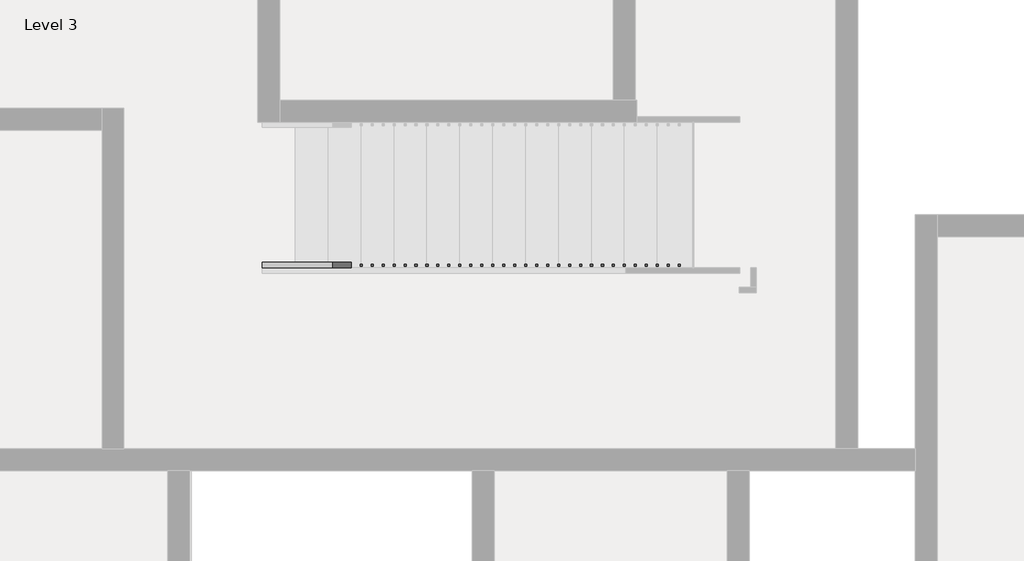
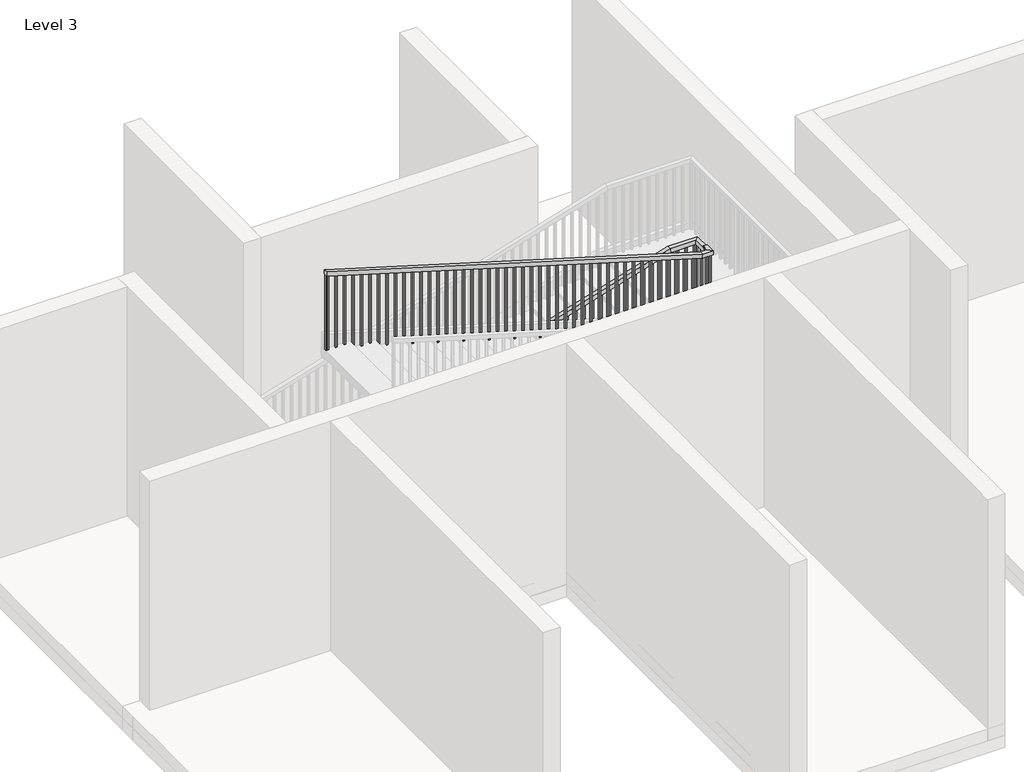
# One storey, part 11 of 14: 1 railing.
"""IFC4 building model written with IfcOpenShell, lengths in millimetres."""

from ifc_helpers import new_model, si_unit, frame, origin, place, context, project, spatial, polyline, outline, extrude, faceted_brep, element, save

model = new_model("IFC4")

# Units and contexts
model_context = context("Model", 3, world=origin())
ifc_project = project(units=[si_unit("LENGTHUNIT", "METRE", prefix="MILLI")], contexts=[model_context])

# Site, building, storey
site = spatial("IfcSite", under=ifc_project)
building = spatial("IfcBuilding", under=site)
storey = spatial("IfcBuildingStorey", under=building, Name="Level 3", Elevation=6096.0)

# Railing
placement = place(None, origin())
element("IfcRailing", 1, ObjectType="Handrail - Rectangular", at=placement, inside=storey, context=model_context, shape_type="SolidModel", body=[
    faceted_brep([(-5254.0891351, 11205.0082924, 7101.84), (-5254.0891351, 11205.0082924, 7048.8032429), (-5254.0891351, 11154.2082924, 7048.8032429), (-5254.0891351, 11154.2082924, 7101.84), (-986.8891351, 11205.0082924, 8382.0), (-979.4332782, 11205.0082924, 8331.2), (-979.4332782, 11154.2082924, 8331.2), (-986.8891351, 11154.2082924, 8382.0), (-631.2891351, 11205.0082924, 8382.0), (-631.2891351, 11205.0082924, 8331.2), (-682.0891351, 11154.2082924, 8331.2), (-682.0891351, 11154.2082924, 8382.0), (-631.2891351, 11001.8082924, 8382.0), (-631.2891351, 10951.0082924, 8331.2), (-682.0891351, 10951.0082924, 8331.2), (-682.0891351, 11001.8082924, 8382.0), (-631.2891351, 11001.8082924, 8404.86), (-631.2891351, 10951.0082924, 8354.06), (-682.0891351, 10951.0082924, 8354.06), (-682.0891351, 11001.8082924, 8404.86), (-631.2891351, 10874.8082924, 8404.86), (-631.2891351, 10874.8082924, 8354.06), (-682.0891351, 10925.6082924, 8354.06), (-682.0891351, 10925.6082924, 8404.86), (-758.2891351, 10874.8082924, 8404.86), (-765.744992, 10874.8082924, 8354.06), (-765.744992, 10925.6082924, 8354.06), (-758.2891351, 10925.6082924, 8404.86), (-5254.0891351, 10874.8082924, 9753.6), (-5254.0891351, 10925.6082924, 9753.6), (-5254.0891351, 10925.6082924, 9700.5632429), (-5254.0891351, 10874.8082924, 9700.5632429)], [[[0, 1, 2, 3]], [[1, 0, 4, 5]], [[2, 1, 5, 6]], [[3, 2, 6, 7]], [[0, 3, 7, 4]], [[5, 4, 8, 9]], [[6, 5, 9, 10]], [[7, 6, 10, 11]], [[4, 7, 11, 8]], [[9, 8, 12, 13]], [[10, 9, 13, 14]], [[11, 10, 14, 15]], [[8, 11, 15, 12]], [[13, 12, 16, 17]], [[14, 13, 17, 18]], [[15, 14, 18, 19]], [[12, 15, 19, 16]], [[17, 16, 20, 21]], [[18, 17, 21, 22]], [[19, 18, 22, 23]], [[16, 19, 23, 20]], [[21, 20, 24, 25]], [[22, 21, 25, 26]], [[23, 22, 26, 27]], [[20, 23, 27, 24]], [[28, 29, 30, 31]], [[25, 24, 28, 31]], [[26, 25, 31, 30]], [[27, 26, 30, 29]], [[24, 27, 29, 28]]]),
    extrude(outline(polyline([(9690.0857429, -5219.1641351), (9695.8007429, -5238.2141351), (8747.76, -5238.2141351), (8747.76, -5219.1641351), (9690.0857429, -5219.1641351)])), frame((0.0, 10890.6832924, 0.0), z_axis=(0.0, 1.0, 0.0), x_axis=(0.0, 0.0, 1.0)), (0.0, 0.0, 1.0), 19.05),
    extrude(outline(polyline([(9659.6057429, -5117.5641351), (9665.3207429, -5136.6141351), (8747.76, -5136.6141351), (8747.76, -5117.5641351), (9659.6057429, -5117.5641351)])), frame((0.0, 10890.6832924, 0.0), z_axis=(0.0, 1.0, 0.0), x_axis=(0.0, 0.0, 1.0)), (0.0, 0.0, 1.0), 19.05),
    extrude(outline(polyline([(9629.1257429, -5015.9641351), (9634.8407429, -5035.0141351), (8747.76, -5035.0141351), (8747.76, -5015.9641351), (9629.1257429, -5015.9641351)])), frame((0.0, 10890.6832924, 0.0), z_axis=(0.0, 1.0, 0.0), x_axis=(0.0, 0.0, 1.0)), (0.0, 0.0, 1.0), 19.05),
    extrude(outline(polyline([(9598.6457429, -4914.3641351), (9604.3607429, -4933.4141351), (8656.32, -4933.4141351), (8656.32, -4914.3641351), (9598.6457429, -4914.3641351)])), frame((0.0, 10890.6832924, 0.0), z_axis=(0.0, 1.0, 0.0), x_axis=(0.0, 0.0, 1.0)), (0.0, 0.0, 1.0), 19.05),
    extrude(outline(polyline([(9568.1657429, -4812.7641351), (9573.8807429, -4831.8141351), (8656.32, -4831.8141351), (8656.32, -4812.7641351), (9568.1657429, -4812.7641351)])), frame((0.0, 10890.6832924, 0.0), z_axis=(0.0, 1.0, 0.0), x_axis=(0.0, 0.0, 1.0)), (0.0, 0.0, 1.0), 19.05),
    extrude(outline(polyline([(9537.6857429, -4711.1641351), (9543.4007429, -4730.2141351), (8656.32, -4730.2141351), (8656.32, -4711.1641351), (9537.6857429, -4711.1641351)])), frame((0.0, 10890.6832924, 0.0), z_axis=(0.0, 1.0, 0.0), x_axis=(0.0, 0.0, 1.0)), (0.0, 0.0, 1.0), 19.05),
    extrude(outline(polyline([(9507.2057429, -4609.5641351), (9512.9207429, -4628.6141351), (8564.88, -4628.6141351), (8564.88, -4609.5641351), (9507.2057429, -4609.5641351)])), frame((0.0, 10890.6832924, 0.0), z_axis=(0.0, 1.0, 0.0), x_axis=(0.0, 0.0, 1.0)), (0.0, 0.0, 1.0), 19.05),
    extrude(outline(polyline([(9476.7257429, -4507.9641351), (9482.4407429, -4527.0141351), (8564.88, -4527.0141351), (8564.88, -4507.9641351), (9476.7257429, -4507.9641351)])), frame((0.0, 10890.6832924, 0.0), z_axis=(0.0, 1.0, 0.0), x_axis=(0.0, 0.0, 1.0)), (0.0, 0.0, 1.0), 19.05),
    extrude(outline(polyline([(9446.2457429, -4406.3641351), (9451.9607429, -4425.4141351), (8564.88, -4425.4141351), (8564.88, -4406.3641351), (9446.2457429, -4406.3641351)])), frame((0.0, 10890.6832924, 0.0), z_axis=(0.0, 1.0, 0.0), x_axis=(0.0, 0.0, 1.0)), (0.0, 0.0, 1.0), 19.05),
    extrude(outline(polyline([(9415.7657429, -4304.7641351), (9421.4807429, -4323.8141351), (8473.44, -4323.8141351), (8473.44, -4304.7641351), (9415.7657429, -4304.7641351)])), frame((0.0, 10890.6832924, 0.0), z_axis=(0.0, 1.0, 0.0), x_axis=(0.0, 0.0, 1.0)), (0.0, 0.0, 1.0), 19.05),
    extrude(outline(polyline([(9385.2857429, -4203.1641351), (9391.0007429, -4222.2141351), (8473.44, -4222.2141351), (8473.44, -4203.1641351), (9385.2857429, -4203.1641351)])), frame((0.0, 10890.6832924, 0.0), z_axis=(0.0, 1.0, 0.0), x_axis=(0.0, 0.0, 1.0)), (0.0, 0.0, 1.0), 19.05),
    extrude(outline(polyline([(9354.8057429, -4101.5641351), (9360.5207429, -4120.6141351), (8473.44, -4120.6141351), (8473.44, -4101.5641351), (9354.8057429, -4101.5641351)])), frame((0.0, 10890.6832924, 0.0), z_axis=(0.0, 1.0, 0.0), x_axis=(0.0, 0.0, 1.0)), (0.0, 0.0, 1.0), 19.05),
    extrude(outline(polyline([(9324.3257429, -3999.9641351), (9330.0407429, -4019.0141351), (8382.0, -4019.0141351), (8382.0, -3999.9641351), (9324.3257429, -3999.9641351)])), frame((0.0, 10890.6832924, 0.0), z_axis=(0.0, 1.0, 0.0), x_axis=(0.0, 0.0, 1.0)), (0.0, 0.0, 1.0), 19.05),
    extrude(outline(polyline([(9293.8457429, -3898.3641351), (9299.5607429, -3917.4141351), (8382.0, -3917.4141351), (8382.0, -3898.3641351), (9293.8457429, -3898.3641351)])), frame((0.0, 10890.6832924, 0.0), z_axis=(0.0, 1.0, 0.0), x_axis=(0.0, 0.0, 1.0)), (0.0, 0.0, 1.0), 19.05),
    extrude(outline(polyline([(9263.3657429, -3796.7641351), (9269.0807429, -3815.8141351), (8382.0, -3815.8141351), (8382.0, -3796.7641351), (9263.3657429, -3796.7641351)])), frame((0.0, 10890.6832924, 0.0), z_axis=(0.0, 1.0, 0.0), x_axis=(0.0, 0.0, 1.0)), (0.0, 0.0, 1.0), 19.05),
    extrude(outline(polyline([(9232.8857429, -3695.1641351), (9238.6007429, -3714.2141351), (8290.56, -3714.2141351), (8290.56, -3695.1641351), (9232.8857429, -3695.1641351)])), frame((0.0, 10890.6832924, 0.0), z_axis=(0.0, 1.0, 0.0), x_axis=(0.0, 0.0, 1.0)), (0.0, 0.0, 1.0), 19.05),
    extrude(outline(polyline([(9202.4057429, -3593.5641351), (9208.1207429, -3612.6141351), (8290.56, -3612.6141351), (8290.56, -3593.5641351), (9202.4057429, -3593.5641351)])), frame((0.0, 10890.6832924, 0.0), z_axis=(0.0, 1.0, 0.0), x_axis=(0.0, 0.0, 1.0)), (0.0, 0.0, 1.0), 19.05),
    extrude(outline(polyline([(9171.9257429, -3491.9641351), (9177.6407429, -3511.0141351), (8290.56, -3511.0141351), (8290.56, -3491.9641351), (9171.9257429, -3491.9641351)])), frame((0.0, 10890.6832924, 0.0), z_axis=(0.0, 1.0, 0.0), x_axis=(0.0, 0.0, 1.0)), (0.0, 0.0, 1.0), 19.05),
    extrude(outline(polyline([(9141.4457429, -3390.3641351), (9147.1607429, -3409.4141351), (8199.12, -3409.4141351), (8199.12, -3390.3641351), (9141.4457429, -3390.3641351)])), frame((0.0, 10890.6832924, 0.0), z_axis=(0.0, 1.0, 0.0), x_axis=(0.0, 0.0, 1.0)), (0.0, 0.0, 1.0), 19.05),
    extrude(outline(polyline([(9110.9657429, -3288.7641351), (9116.6807429, -3307.8141351), (8199.12, -3307.8141351), (8199.12, -3288.7641351), (9110.9657429, -3288.7641351)])), frame((0.0, 10890.6832924, 0.0), z_axis=(0.0, 1.0, 0.0), x_axis=(0.0, 0.0, 1.0)), (0.0, 0.0, 1.0), 19.05),
    extrude(outline(polyline([(9080.4857429, -3187.1641351), (9086.2007429, -3206.2141351), (8199.12, -3206.2141351), (8199.12, -3187.1641351), (9080.4857429, -3187.1641351)])), frame((0.0, 10890.6832924, 0.0), z_axis=(0.0, 1.0, 0.0), x_axis=(0.0, 0.0, 1.0)), (0.0, 0.0, 1.0), 19.05),
    extrude(outline(polyline([(9050.0057429, -3085.5641351), (9055.7207429, -3104.6141351), (8107.68, -3104.6141351), (8107.68, -3085.5641351), (9050.0057429, -3085.5641351)])), frame((0.0, 10890.6832924, 0.0), z_axis=(0.0, 1.0, 0.0), x_axis=(0.0, 0.0, 1.0)), (0.0, 0.0, 1.0), 19.05),
    extrude(outline(polyline([(9019.5257429, -2983.9641351), (9025.2407429, -3003.0141351), (8107.68, -3003.0141351), (8107.68, -2983.9641351), (9019.5257429, -2983.9641351)])), frame((0.0, 10890.6832924, 0.0), z_axis=(0.0, 1.0, 0.0), x_axis=(0.0, 0.0, 1.0)), (0.0, 0.0, 1.0), 19.05),
    extrude(outline(polyline([(8989.0457429, -2882.3641351), (8994.7607429, -2901.4141351), (8107.68, -2901.4141351), (8107.68, -2882.3641351), (8989.0457429, -2882.3641351)])), frame((0.0, 10890.6832924, 0.0), z_axis=(0.0, 1.0, 0.0), x_axis=(0.0, 0.0, 1.0)), (0.0, 0.0, 1.0), 19.05),
    extrude(outline(polyline([(8958.5657429, -2780.7641351), (8964.2807429, -2799.8141351), (8016.24, -2799.8141351), (8016.24, -2780.7641351), (8958.5657429, -2780.7641351)])), frame((0.0, 10890.6832924, 0.0), z_axis=(0.0, 1.0, 0.0), x_axis=(0.0, 0.0, 1.0)), (0.0, 0.0, 1.0), 19.05),
    extrude(outline(polyline([(8928.0857429, -2679.1641351), (8933.8007429, -2698.2141351), (8016.24, -2698.2141351), (8016.24, -2679.1641351), (8928.0857429, -2679.1641351)])), frame((0.0, 10890.6832924, 0.0), z_axis=(0.0, 1.0, 0.0), x_axis=(0.0, 0.0, 1.0)), (0.0, 0.0, 1.0), 19.05),
    extrude(outline(polyline([(8897.6057429, -2577.5641351), (8903.3207429, -2596.6141351), (8016.24, -2596.6141351), (8016.24, -2577.5641351), (8897.6057429, -2577.5641351)])), frame((0.0, 10890.6832924, 0.0), z_axis=(0.0, 1.0, 0.0), x_axis=(0.0, 0.0, 1.0)), (0.0, 0.0, 1.0), 19.05),
    extrude(outline(polyline([(8867.1257429, -2475.9641351), (8872.8407429, -2495.0141351), (7924.8, -2495.0141351), (7924.8, -2475.9641351), (8867.1257429, -2475.9641351)])), frame((0.0, 10890.6832924, 0.0), z_axis=(0.0, 1.0, 0.0), x_axis=(0.0, 0.0, 1.0)), (0.0, 0.0, 1.0), 19.05),
    extrude(outline(polyline([(8836.6457429, -2374.3641351), (8842.3607429, -2393.4141351), (7924.8, -2393.4141351), (7924.8, -2374.3641351), (8836.6457429, -2374.3641351)])), frame((0.0, 10890.6832924, 0.0), z_axis=(0.0, 1.0, 0.0), x_axis=(0.0, 0.0, 1.0)), (0.0, 0.0, 1.0), 19.05),
    extrude(outline(polyline([(8806.1657429, -2272.7641351), (8811.8807429, -2291.8141351), (7924.8, -2291.8141351), (7924.8, -2272.7641351), (8806.1657429, -2272.7641351)])), frame((0.0, 10890.6832924, 0.0), z_axis=(0.0, 1.0, 0.0), x_axis=(0.0, 0.0, 1.0)), (0.0, 0.0, 1.0), 19.05),
    extrude(outline(polyline([(8775.6857429, -2171.1641351), (8781.4007429, -2190.2141351), (7833.36, -2190.2141351), (7833.36, -2171.1641351), (8775.6857429, -2171.1641351)])), frame((0.0, 10890.6832924, 0.0), z_axis=(0.0, 1.0, 0.0), x_axis=(0.0, 0.0, 1.0)), (0.0, 0.0, 1.0), 19.05),
    extrude(outline(polyline([(8745.2057429, -2069.5641351), (8750.9207429, -2088.6141351), (7833.36, -2088.6141351), (7833.36, -2069.5641351), (8745.2057429, -2069.5641351)])), frame((0.0, 10890.6832924, 0.0), z_axis=(0.0, 1.0, 0.0), x_axis=(0.0, 0.0, 1.0)), (0.0, 0.0, 1.0), 19.05),
    extrude(outline(polyline([(8714.7257429, -1967.9641351), (8720.4407429, -1987.0141351), (7833.36, -1987.0141351), (7833.36, -1967.9641351), (8714.7257429, -1967.9641351)])), frame((0.0, 10890.6832924, 0.0), z_axis=(0.0, 1.0, 0.0), x_axis=(0.0, 0.0, 1.0)), (0.0, 0.0, 1.0), 19.05),
    extrude(outline(polyline([(8684.2457429, -1866.3641351), (8689.9607429, -1885.4141351), (7741.92, -1885.4141351), (7741.92, -1866.3641351), (8684.2457429, -1866.3641351)])), frame((0.0, 10890.6832924, 0.0), z_axis=(0.0, 1.0, 0.0), x_axis=(0.0, 0.0, 1.0)), (0.0, 0.0, 1.0), 19.05),
    extrude(outline(polyline([(8653.7657429, -1764.7641351), (8659.4807429, -1783.8141351), (7741.92, -1783.8141351), (7741.92, -1764.7641351), (8653.7657429, -1764.7641351)])), frame((0.0, 10890.6832924, 0.0), z_axis=(0.0, 1.0, 0.0), x_axis=(0.0, 0.0, 1.0)), (0.0, 0.0, 1.0), 19.05),
    extrude(outline(polyline([(8623.2857429, -1663.1641351), (8629.0007429, -1682.2141351), (7741.92, -1682.2141351), (7741.92, -1663.1641351), (8623.2857429, -1663.1641351)])), frame((0.0, 10890.6832924, 0.0), z_axis=(0.0, 1.0, 0.0), x_axis=(0.0, 0.0, 1.0)), (0.0, 0.0, 1.0), 19.05),
    extrude(outline(polyline([(8592.8057429, -1561.5641351), (8598.5207429, -1580.6141351), (7650.48, -1580.6141351), (7650.48, -1561.5641351), (8592.8057429, -1561.5641351)])), frame((0.0, 10890.6832924, 0.0), z_axis=(0.0, 1.0, 0.0), x_axis=(0.0, 0.0, 1.0)), (0.0, 0.0, 1.0), 19.05),
    extrude(outline(polyline([(8562.3257429, -1459.9641351), (8568.0407429, -1479.0141351), (7650.48, -1479.0141351), (7650.48, -1459.9641351), (8562.3257429, -1459.9641351)])), frame((0.0, 10890.6832924, 0.0), z_axis=(0.0, 1.0, 0.0), x_axis=(0.0, 0.0, 1.0)), (0.0, 0.0, 1.0), 19.05),
    extrude(outline(polyline([(8531.8457429, -1358.3641351), (8537.5607429, -1377.4141351), (7650.48, -1377.4141351), (7650.48, -1358.3641351), (8531.8457429, -1358.3641351)])), frame((0.0, 10890.6832924, 0.0), z_axis=(0.0, 1.0, 0.0), x_axis=(0.0, 0.0, 1.0)), (0.0, 0.0, 1.0), 19.05),
    extrude(outline(polyline([(8501.3657429, -1256.7641351), (8507.0807429, -1275.8141351), (7559.04, -1275.8141351), (7559.04, -1256.7641351), (8501.3657429, -1256.7641351)])), frame((0.0, 10890.6832924, 0.0), z_axis=(0.0, 1.0, 0.0), x_axis=(0.0, 0.0, 1.0)), (0.0, 0.0, 1.0), 19.05),
    extrude(outline(polyline([(8470.8857429, -1155.1641351), (8476.6007429, -1174.2141351), (7559.04, -1174.2141351), (7559.04, -1155.1641351), (8470.8857429, -1155.1641351)])), frame((0.0, 10890.6832924, 0.0), z_axis=(0.0, 1.0, 0.0), x_axis=(0.0, 0.0, 1.0)), (0.0, 0.0, 1.0), 19.05),
    extrude(outline(polyline([(8440.4057429, -1053.5641351), (8446.1207429, -1072.6141351), (7559.04, -1072.6141351), (7559.04, -1053.5641351), (8440.4057429, -1053.5641351)])), frame((0.0, 10890.6832924, 0.0), z_axis=(0.0, 1.0, 0.0), x_axis=(0.0, 0.0, 1.0)), (0.0, 0.0, 1.0), 19.05),
    extrude(outline(polyline([(8409.9257429, -951.9641351), (8415.6407429, -971.0141351), (7467.6, -971.0141351), (7467.6, -951.9641351), (8409.9257429, -951.9641351)])), frame((0.0, 10890.6832924, 0.0), z_axis=(0.0, 1.0, 0.0), x_axis=(0.0, 0.0, 1.0)), (0.0, 0.0, 1.0), 19.05),
    extrude(outline(polyline([(8379.4457429, -850.3641351), (8385.1607429, -869.4141351), (7467.6, -869.4141351), (7467.6, -850.3641351), (8379.4457429, -850.3641351)])), frame((0.0, 10890.6832924, 0.0), z_axis=(0.0, 1.0, 0.0), x_axis=(0.0, 0.0, 1.0)), (0.0, 0.0, 1.0), 19.05),
    extrude(outline(polyline([(8348.9657429, -748.7641351), (8354.6807429, -767.8141351), (7467.6, -767.8141351), (7467.6, -748.7641351), (8348.9657429, -748.7641351)])), frame((0.0, 10890.6832924, 0.0), z_axis=(0.0, 1.0, 0.0), x_axis=(0.0, 0.0, 1.0)), (0.0, 0.0, 1.0), 19.05),
    extrude(outline(polyline([(-666.2141351, 10985.9332924), (-647.1641351, 10985.9332924), (-647.1641351, 10966.8832924), (-666.2141351, 10966.8832924), (-666.2141351, 10985.9332924)])), frame((0.0, 0.0, 7467.6), z_axis=(0.0, 0.0, 1.0), x_axis=(1.0, 0.0, 0.0)), (0.0, 0.0, 1.0), 886.46),
    extrude(outline(polyline([(-666.2141351, 11087.5332924), (-647.1641351, 11087.5332924), (-647.1641351, 11068.4832924), (-666.2141351, 11068.4832924), (-666.2141351, 11087.5332924)])), frame((0.0, 0.0, 7467.6), z_axis=(0.0, 0.0, 1.0), x_axis=(1.0, 0.0, 0.0)), (0.0, 0.0, 1.0), 863.6),
    extrude(outline(polyline([(-691.6141351, 11170.0832924), (-691.6141351, 11189.1332924), (-672.5641351, 11189.1332924), (-672.5641351, 11170.0832924), (-691.6141351, 11170.0832924)])), frame((0.0, 0.0, 7467.6), z_axis=(0.0, 0.0, 1.0), x_axis=(1.0, 0.0, 0.0)), (0.0, 0.0, 1.0), 863.6),
    extrude(outline(polyline([(-793.2141351, 11170.0832924), (-793.2141351, 11189.1332924), (-774.1641351, 11189.1332924), (-774.1641351, 11170.0832924), (-793.2141351, 11170.0832924)])), frame((0.0, 0.0, 7467.6), z_axis=(0.0, 0.0, 1.0), x_axis=(1.0, 0.0, 0.0)), (0.0, 0.0, 1.0), 863.6),
    extrude(outline(polyline([(-894.8141351, 11170.0832924), (-894.8141351, 11189.1332924), (-875.7641351, 11189.1332924), (-875.7641351, 11170.0832924), (-894.8141351, 11170.0832924)])), frame((0.0, 0.0, 7467.6), z_axis=(0.0, 0.0, 1.0), x_axis=(1.0, 0.0, 0.0)), (0.0, 0.0, 1.0), 863.6),
    extrude(outline(polyline([(8331.8207429, -977.3641351), (8326.1057429, -996.4141351), (7467.6, -996.4141351), (7467.6, -977.3641351), (8331.8207429, -977.3641351)])), frame((0.0, 11170.0832924, 0.0), z_axis=(0.0, 1.0, 0.0), x_axis=(0.0, 0.0, 1.0)), (0.0, 0.0, 1.0), 19.05),
    extrude(outline(polyline([(8301.3407429, -1078.9641351), (8295.6257429, -1098.0141351), (7376.16, -1098.0141351), (7376.16, -1078.9641351), (8301.3407429, -1078.9641351)])), frame((0.0, 11170.0832924, 0.0), z_axis=(0.0, 1.0, 0.0), x_axis=(0.0, 0.0, 1.0)), (0.0, 0.0, 1.0), 19.05),
    extrude(outline(polyline([(8270.8607429, -1180.5641351), (8265.1457429, -1199.6141351), (7376.16, -1199.6141351), (7376.16, -1180.5641351), (8270.8607429, -1180.5641351)])), frame((0.0, 11170.0832924, 0.0), z_axis=(0.0, 1.0, 0.0), x_axis=(0.0, 0.0, 1.0)), (0.0, 0.0, 1.0), 19.05),
    extrude(outline(polyline([(8240.3807429, -1282.1641351), (8234.6657429, -1301.2141351), (7376.16, -1301.2141351), (7376.16, -1282.1641351), (8240.3807429, -1282.1641351)])), frame((0.0, 11170.0832924, 0.0), z_axis=(0.0, 1.0, 0.0), x_axis=(0.0, 0.0, 1.0)), (0.0, 0.0, 1.0), 19.05),
    extrude(outline(polyline([(8209.9007429, -1383.7641351), (8204.1857429, -1402.8141351), (7284.72, -1402.8141351), (7284.72, -1383.7641351), (8209.9007429, -1383.7641351)])), frame((0.0, 11170.0832924, 0.0), z_axis=(0.0, 1.0, 0.0), x_axis=(0.0, 0.0, 1.0)), (0.0, 0.0, 1.0), 19.05),
    extrude(outline(polyline([(8179.4207429, -1485.3641351), (8173.7057429, -1504.4141351), (7284.72, -1504.4141351), (7284.72, -1485.3641351), (8179.4207429, -1485.3641351)])), frame((0.0, 11170.0832924, 0.0), z_axis=(0.0, 1.0, 0.0), x_axis=(0.0, 0.0, 1.0)), (0.0, 0.0, 1.0), 19.05),
    extrude(outline(polyline([(8148.9407429, -1586.9641351), (8143.2257429, -1606.0141351), (7284.72, -1606.0141351), (7284.72, -1586.9641351), (8148.9407429, -1586.9641351)])), frame((0.0, 11170.0832924, 0.0), z_axis=(0.0, 1.0, 0.0), x_axis=(0.0, 0.0, 1.0)), (0.0, 0.0, 1.0), 19.05),
    extrude(outline(polyline([(8118.4607429, -1688.5641351), (8112.7457429, -1707.6141351), (7193.28, -1707.6141351), (7193.28, -1688.5641351), (8118.4607429, -1688.5641351)])), frame((0.0, 11170.0832924, 0.0), z_axis=(0.0, 1.0, 0.0), x_axis=(0.0, 0.0, 1.0)), (0.0, 0.0, 1.0), 19.05),
    extrude(outline(polyline([(8087.9807429, -1790.1641351), (8082.2657429, -1809.2141351), (7193.28, -1809.2141351), (7193.28, -1790.1641351), (8087.9807429, -1790.1641351)])), frame((0.0, 11170.0832924, 0.0), z_axis=(0.0, 1.0, 0.0), x_axis=(0.0, 0.0, 1.0)), (0.0, 0.0, 1.0), 19.05),
    extrude(outline(polyline([(8057.5007429, -1891.7641351), (8051.7857429, -1910.8141351), (7193.28, -1910.8141351), (7193.28, -1891.7641351), (8057.5007429, -1891.7641351)])), frame((0.0, 11170.0832924, 0.0), z_axis=(0.0, 1.0, 0.0), x_axis=(0.0, 0.0, 1.0)), (0.0, 0.0, 1.0), 19.05),
    extrude(outline(polyline([(8027.0207429, -1993.3641351), (8021.3057429, -2012.4141351), (7101.84, -2012.4141351), (7101.84, -1993.3641351), (8027.0207429, -1993.3641351)])), frame((0.0, 11170.0832924, 0.0), z_axis=(0.0, 1.0, 0.0), x_axis=(0.0, 0.0, 1.0)), (0.0, 0.0, 1.0), 19.05),
    extrude(outline(polyline([(7996.5407429, -2094.9641351), (7990.8257429, -2114.0141351), (7101.84, -2114.0141351), (7101.84, -2094.9641351), (7996.5407429, -2094.9641351)])), frame((0.0, 11170.0832924, 0.0), z_axis=(0.0, 1.0, 0.0), x_axis=(0.0, 0.0, 1.0)), (0.0, 0.0, 1.0), 19.05),
    extrude(outline(polyline([(7966.0607429, -2196.5641351), (7960.3457429, -2215.6141351), (7101.84, -2215.6141351), (7101.84, -2196.5641351), (7966.0607429, -2196.5641351)])), frame((0.0, 11170.0832924, 0.0), z_axis=(0.0, 1.0, 0.0), x_axis=(0.0, 0.0, 1.0)), (0.0, 0.0, 1.0), 19.05),
    extrude(outline(polyline([(7935.5807429, -2298.1641351), (7929.8657429, -2317.2141351), (7010.4, -2317.2141351), (7010.4, -2298.1641351), (7935.5807429, -2298.1641351)])), frame((0.0, 11170.0832924, 0.0), z_axis=(0.0, 1.0, 0.0), x_axis=(0.0, 0.0, 1.0)), (0.0, 0.0, 1.0), 19.05),
    extrude(outline(polyline([(7905.1007429, -2399.7641351), (7899.3857429, -2418.8141351), (7010.4, -2418.8141351), (7010.4, -2399.7641351), (7905.1007429, -2399.7641351)])), frame((0.0, 11170.0832924, 0.0), z_axis=(0.0, 1.0, 0.0), x_axis=(0.0, 0.0, 1.0)), (0.0, 0.0, 1.0), 19.05),
    extrude(outline(polyline([(7874.6207429, -2501.3641351), (7868.9057429, -2520.4141351), (7010.4, -2520.4141351), (7010.4, -2501.3641351), (7874.6207429, -2501.3641351)])), frame((0.0, 11170.0832924, 0.0), z_axis=(0.0, 1.0, 0.0), x_axis=(0.0, 0.0, 1.0)), (0.0, 0.0, 1.0), 19.05),
    extrude(outline(polyline([(7844.1407429, -2602.9641351), (7838.4257429, -2622.0141351), (6918.96, -2622.0141351), (6918.96, -2602.9641351), (7844.1407429, -2602.9641351)])), frame((0.0, 11170.0832924, 0.0), z_axis=(0.0, 1.0, 0.0), x_axis=(0.0, 0.0, 1.0)), (0.0, 0.0, 1.0), 19.05),
    extrude(outline(polyline([(7813.6607429, -2704.5641351), (7807.9457429, -2723.6141351), (6918.96, -2723.6141351), (6918.96, -2704.5641351), (7813.6607429, -2704.5641351)])), frame((0.0, 11170.0832924, 0.0), z_axis=(0.0, 1.0, 0.0), x_axis=(0.0, 0.0, 1.0)), (0.0, 0.0, 1.0), 19.05),
    extrude(outline(polyline([(7783.1807429, -2806.1641351), (7777.4657429, -2825.2141351), (6918.96, -2825.2141351), (6918.96, -2806.1641351), (7783.1807429, -2806.1641351)])), frame((0.0, 11170.0832924, 0.0), z_axis=(0.0, 1.0, 0.0), x_axis=(0.0, 0.0, 1.0)), (0.0, 0.0, 1.0), 19.05),
    extrude(outline(polyline([(7752.7007429, -2907.7641351), (7746.9857429, -2926.8141351), (6827.52, -2926.8141351), (6827.52, -2907.7641351), (7752.7007429, -2907.7641351)])), frame((0.0, 11170.0832924, 0.0), z_axis=(0.0, 1.0, 0.0), x_axis=(0.0, 0.0, 1.0)), (0.0, 0.0, 1.0), 19.05),
    extrude(outline(polyline([(7722.2207429, -3009.3641351), (7716.5057429, -3028.4141351), (6827.52, -3028.4141351), (6827.52, -3009.3641351), (7722.2207429, -3009.3641351)])), frame((0.0, 11170.0832924, 0.0), z_axis=(0.0, 1.0, 0.0), x_axis=(0.0, 0.0, 1.0)), (0.0, 0.0, 1.0), 19.05),
    extrude(outline(polyline([(7691.7407429, -3110.9641351), (7686.0257429, -3130.0141351), (6827.52, -3130.0141351), (6827.52, -3110.9641351), (7691.7407429, -3110.9641351)])), frame((0.0, 11170.0832924, 0.0), z_axis=(0.0, 1.0, 0.0), x_axis=(0.0, 0.0, 1.0)), (0.0, 0.0, 1.0), 19.05),
    extrude(outline(polyline([(7661.2607429, -3212.5641351), (7655.5457429, -3231.6141351), (6736.08, -3231.6141351), (6736.08, -3212.5641351), (7661.2607429, -3212.5641351)])), frame((0.0, 11170.0832924, 0.0), z_axis=(0.0, 1.0, 0.0), x_axis=(0.0, 0.0, 1.0)), (0.0, 0.0, 1.0), 19.05),
    extrude(outline(polyline([(7630.7807429, -3314.1641351), (7625.0657429, -3333.2141351), (6736.08, -3333.2141351), (6736.08, -3314.1641351), (7630.7807429, -3314.1641351)])), frame((0.0, 11170.0832924, 0.0), z_axis=(0.0, 1.0, 0.0), x_axis=(0.0, 0.0, 1.0)), (0.0, 0.0, 1.0), 19.05),
    extrude(outline(polyline([(7600.3007429, -3415.7641351), (7594.5857429, -3434.8141351), (6736.08, -3434.8141351), (6736.08, -3415.7641351), (7600.3007429, -3415.7641351)])), frame((0.0, 11170.0832924, 0.0), z_axis=(0.0, 1.0, 0.0), x_axis=(0.0, 0.0, 1.0)), (0.0, 0.0, 1.0), 19.05),
    extrude(outline(polyline([(7569.8207429, -3517.3641351), (7564.1057429, -3536.4141351), (6644.64, -3536.4141351), (6644.64, -3517.3641351), (7569.8207429, -3517.3641351)])), frame((0.0, 11170.0832924, 0.0), z_axis=(0.0, 1.0, 0.0), x_axis=(0.0, 0.0, 1.0)), (0.0, 0.0, 1.0), 19.05),
    extrude(outline(polyline([(7539.3407429, -3618.9641351), (7533.6257429, -3638.0141351), (6644.64, -3638.0141351), (6644.64, -3618.9641351), (7539.3407429, -3618.9641351)])), frame((0.0, 11170.0832924, 0.0), z_axis=(0.0, 1.0, 0.0), x_axis=(0.0, 0.0, 1.0)), (0.0, 0.0, 1.0), 19.05),
    extrude(outline(polyline([(7508.8607429, -3720.5641351), (7503.1457429, -3739.6141351), (6644.64, -3739.6141351), (6644.64, -3720.5641351), (7508.8607429, -3720.5641351)])), frame((0.0, 11170.0832924, 0.0), z_axis=(0.0, 1.0, 0.0), x_axis=(0.0, 0.0, 1.0)), (0.0, 0.0, 1.0), 19.05),
    extrude(outline(polyline([(7478.3807429, -3822.1641351), (7472.6657429, -3841.2141351), (6553.2, -3841.2141351), (6553.2, -3822.1641351), (7478.3807429, -3822.1641351)])), frame((0.0, 11170.0832924, 0.0), z_axis=(0.0, 1.0, 0.0), x_axis=(0.0, 0.0, 1.0)), (0.0, 0.0, 1.0), 19.05),
    extrude(outline(polyline([(7447.9007429, -3923.7641351), (7442.1857429, -3942.8141351), (6553.2, -3942.8141351), (6553.2, -3923.7641351), (7447.9007429, -3923.7641351)])), frame((0.0, 11170.0832924, 0.0), z_axis=(0.0, 1.0, 0.0), x_axis=(0.0, 0.0, 1.0)), (0.0, 0.0, 1.0), 19.05),
    extrude(outline(polyline([(7417.4207429, -4025.3641351), (7411.7057429, -4044.4141351), (6553.2, -4044.4141351), (6553.2, -4025.3641351), (7417.4207429, -4025.3641351)])), frame((0.0, 11170.0832924, 0.0), z_axis=(0.0, 1.0, 0.0), x_axis=(0.0, 0.0, 1.0)), (0.0, 0.0, 1.0), 19.05),
    extrude(outline(polyline([(7386.9407429, -4126.9641351), (7381.2257429, -4146.0141351), (6461.76, -4146.0141351), (6461.76, -4126.9641351), (7386.9407429, -4126.9641351)])), frame((0.0, 11170.0832924, 0.0), z_axis=(0.0, 1.0, 0.0), x_axis=(0.0, 0.0, 1.0)), (0.0, 0.0, 1.0), 19.05),
    extrude(outline(polyline([(7356.4607429, -4228.5641351), (7350.7457429, -4247.6141351), (6461.76, -4247.6141351), (6461.76, -4228.5641351), (7356.4607429, -4228.5641351)])), frame((0.0, 11170.0832924, 0.0), z_axis=(0.0, 1.0, 0.0), x_axis=(0.0, 0.0, 1.0)), (0.0, 0.0, 1.0), 19.05),
    extrude(outline(polyline([(7325.9807429, -4330.1641351), (7320.2657429, -4349.2141351), (6461.76, -4349.2141351), (6461.76, -4330.1641351), (7325.9807429, -4330.1641351)])), frame((0.0, 11170.0832924, 0.0), z_axis=(0.0, 1.0, 0.0), x_axis=(0.0, 0.0, 1.0)), (0.0, 0.0, 1.0), 19.05),
    extrude(outline(polyline([(7295.5007429, -4431.7641351), (7289.7857429, -4450.8141351), (6370.32, -4450.8141351), (6370.32, -4431.7641351), (7295.5007429, -4431.7641351)])), frame((0.0, 11170.0832924, 0.0), z_axis=(0.0, 1.0, 0.0), x_axis=(0.0, 0.0, 1.0)), (0.0, 0.0, 1.0), 19.05),
    extrude(outline(polyline([(7265.0207429, -4533.3641351), (7259.3057429, -4552.4141351), (6370.32, -4552.4141351), (6370.32, -4533.3641351), (7265.0207429, -4533.3641351)])), frame((0.0, 11170.0832924, 0.0), z_axis=(0.0, 1.0, 0.0), x_axis=(0.0, 0.0, 1.0)), (0.0, 0.0, 1.0), 19.05),
    extrude(outline(polyline([(7234.5407429, -4634.9641351), (7228.8257429, -4654.0141351), (6370.32, -4654.0141351), (6370.32, -4634.9641351), (7234.5407429, -4634.9641351)])), frame((0.0, 11170.0832924, 0.0), z_axis=(0.0, 1.0, 0.0), x_axis=(0.0, 0.0, 1.0)), (0.0, 0.0, 1.0), 19.05),
    extrude(outline(polyline([(7204.0607429, -4736.5641351), (7198.3457429, -4755.6141351), (6278.88, -4755.6141351), (6278.88, -4736.5641351), (7204.0607429, -4736.5641351)])), frame((0.0, 11170.0832924, 0.0), z_axis=(0.0, 1.0, 0.0), x_axis=(0.0, 0.0, 1.0)), (0.0, 0.0, 1.0), 19.05),
    extrude(outline(polyline([(7173.5807429, -4838.1641351), (7167.8657429, -4857.2141351), (6278.88, -4857.2141351), (6278.88, -4838.1641351), (7173.5807429, -4838.1641351)])), frame((0.0, 11170.0832924, 0.0), z_axis=(0.0, 1.0, 0.0), x_axis=(0.0, 0.0, 1.0)), (0.0, 0.0, 1.0), 19.05),
    extrude(outline(polyline([(7143.1007429, -4939.7641351), (7137.3857429, -4958.8141351), (6278.88, -4958.8141351), (6278.88, -4939.7641351), (7143.1007429, -4939.7641351)])), frame((0.0, 11170.0832924, 0.0), z_axis=(0.0, 1.0, 0.0), x_axis=(0.0, 0.0, 1.0)), (0.0, 0.0, 1.0), 19.05),
    extrude(outline(polyline([(7112.6207429, -5041.3641351), (7106.9057429, -5060.4141351), (6187.44, -5060.4141351), (6187.44, -5041.3641351), (7112.6207429, -5041.3641351)])), frame((0.0, 11170.0832924, 0.0), z_axis=(0.0, 1.0, 0.0), x_axis=(0.0, 0.0, 1.0)), (0.0, 0.0, 1.0), 19.05),
    extrude(outline(polyline([(7082.1407429, -5142.9641351), (7076.4257429, -5162.0141351), (6187.44, -5162.0141351), (6187.44, -5142.9641351), (7082.1407429, -5142.9641351)])), frame((0.0, 11170.0832924, 0.0), z_axis=(0.0, 1.0, 0.0), x_axis=(0.0, 0.0, 1.0)), (0.0, 0.0, 1.0), 19.05),
    extrude(outline(polyline([(-666.2141351, 10909.7332924), (-647.1641351, 10909.7332924), (-647.1641351, 10890.6832924), (-666.2141351, 10890.6832924), (-666.2141351, 10909.7332924)])), frame((0.0, 0.0, 7467.6), z_axis=(0.0, 0.0, 1.0), x_axis=(1.0, 0.0, 0.0)), (0.0, 0.0, 1.0), 886.46),
    extrude(outline(polyline([(-666.2141351, 11170.0832924), (-666.2141351, 11189.1332924), (-647.1641351, 11189.1332924), (-647.1641351, 11170.0832924), (-666.2141351, 11170.0832924)])), frame((0.0, 0.0, 7467.6), z_axis=(0.0, 0.0, 1.0), x_axis=(1.0, 0.0, 0.0)), (0.0, 0.0, 1.0), 863.6),
    extrude(outline(polyline([(9694.8482429, -5235.0391351), (9700.5632429, -5254.0891351), (8747.76, -5254.0891351), (8747.76, -5235.0391351), (9694.8482429, -5235.0391351)])), frame((0.0, 10890.6832924, 0.0), z_axis=(0.0, 1.0, 0.0), x_axis=(0.0, 0.0, 1.0)), (0.0, 0.0, 1.0), 19.05),
    extrude(outline(polyline([(7054.5182429, -5235.0391351), (7048.8032429, -5254.0891351), (6187.44, -5254.0891351), (6187.44, -5235.0391351), (7054.5182429, -5235.0391351)])), frame((0.0, 11170.0832924, 0.0), z_axis=(0.0, 1.0, 0.0), x_axis=(0.0, 0.0, 1.0)), (0.0, 0.0, 1.0), 19.05),
])

save(model, "model.ifc")

# Revit data of these elements
# Type "Handrail - Rectangular"
#   Assembly Code = "C2010400"
#   built-in parameter 1008612 = 0.0416667 (stored number, unit not read)
#   built-in parameter 1008611 = 0.0416667 (stored number, unit not read)
#   built-in parameter 1008609 = 0.333333 (stored number, unit not read)
#   built-in parameter 1008604 = 0.166667 (stored number, unit not read)
#   built-in parameter 1008603 = 0.166667 (stored number, unit not read)
#   Railing Height = 3' - 0"
#   built-in parameter 1008630 = 2
#   built-in parameter 1008610 = 2
#   built-in parameter 1008618 = Baluster - Square : 3/4"
# Element 1 (IfcRailing, "Handrail - Rectangular")
#   Phase Created = New Construction
